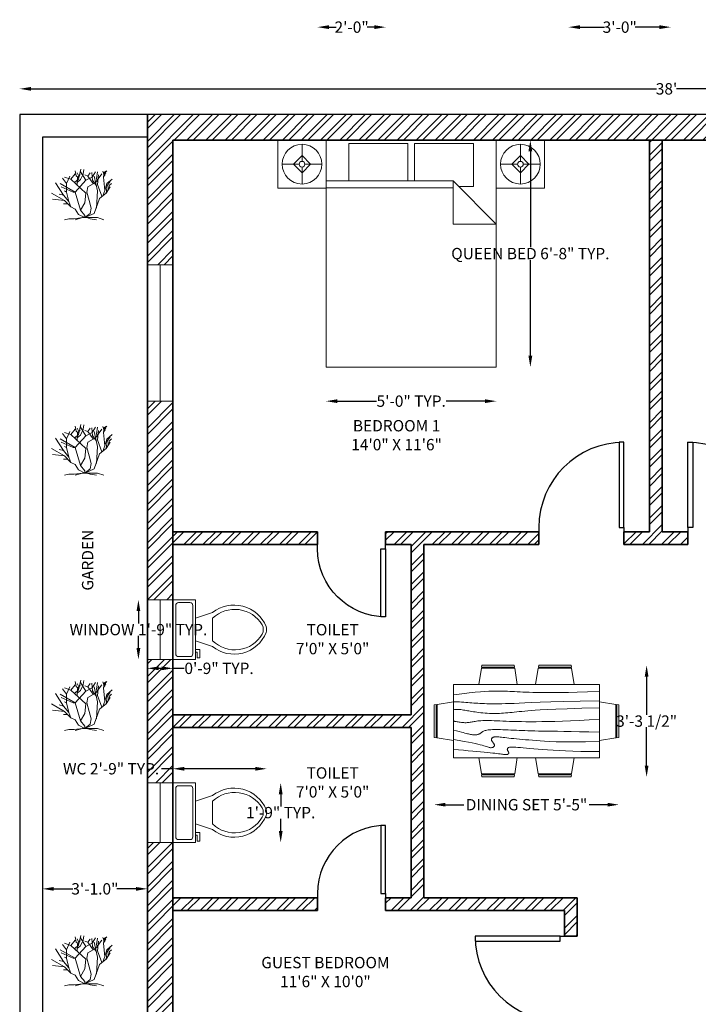
# Model space of a CAD drawing. Units: inches. Extents: x 0 to 478, y -33 to 633.
# Tile 3 of 4: x 0 to 239, y 286 to 633. Entities that reach past the tile are written whole.
import ezdxf

# ---------------------------------------------------------------- set-up
doc = ezdxf.new("R2010")
doc.units = ezdxf.units.IN
for name, color, linetype, lineweight in [('A-ANNO-DIMS', 2, 'Continuous', 18), ('A-AREA-IDEN', 7, 'Continuous', 18), ('A-DOOR', 3, 'Continuous', 25), ('A-FLOR-FIXT', 9, 'Continuous', 18), ('A-FURN', 8, 'Continuous', 18), ('A-GLAZ', 4, 'Continuous', 18), ('A-WALL', 7, 'Continuous', 35), ('A-WALL-PATT', 252, 'Continuous', 13), ('C-PROP', 7, 'Continuous', 30), ('L-PLNT', 3, 'Continuous', 18)]:
    doc.layers.add(name, color=color, linetype=linetype, lineweight=lineweight)
doc.styles.get("Standard").update_dxf_attribs({"font": 'arial.ttf'})
doc.dimstyles.get("Standard").update_dxf_attribs({"dimtxt": 4, "dimasz": 4, "dimexe": 0.18, "dimexo": 0.0625, "dimgap": 0.09, "dimtad": 0, "dimtih": 1, "dimtoh": 1, "dimdec": 1, "dimzin": 0, "dimdsep": 46, "dimlunit": 3, "dimtxsty": 'Standard', "dimcen": 0.09, "dimse1": 1, "dimse2": 1, "dimadec": 0, "dimazin": 0, "dimtfac": 1, "dimtdec": 1, "dimtofl": 0, "dimtmove": 0, "dimatfit": 3, "dimfxl": 1, "dimtolj": 1, "dimtzin": 0, "dimarcsym": 0})

# ---------------------------------------------------------------- blocks, each defined once
blk = doc.blocks.new('Dining Set - 36 x 72 in.')
for p, q in [((-22.2343, 26.00059), (-23.4847, 17.99762)), ((-22.2304, 26), (-5.7608, 26)), ((-22, 27.5), (-22.1562, 26.50042)), ((-5.8416, 26.5), (-22.1534, 26.5)), ((-22, 27.5), (-6, 27.5)), ((-5.8437, 26.49966), (-6, 27.5)), ((-4.5152, 17.99762), (-5.7655, 25.99926)), ((5.7657, 26.00059), (4.5153, 17.99762)), ((5.7696, 26), (22.2392, 26)), ((6, 27.5), (5.8438, 26.50042)), ((22.1584, 26.5), (5.8466, 26.5)), ((6, 27.5), (22, 27.5)), ((22.1563, 26.49966), (22, 27.5)), ((23.4848, 17.99762), (22.2345, 25.99926)), ((36, 18), (-36, 18)), ((-36, 18), (-36, -18)), ((36, -18), (36, 18)), ((-45.5, 8), (-44.5004, 8.15617)), ((-45.5, 8), (-45.5, -8)), ((-44.5, -8.15843), (-44.5, 8.15338)), ((-44.0006, 8.23428), (-35.9976, 9.48474)), ((-44, 8.23041), (-44, -8.23915)), ((44.0006, 8.23428), (35.9976, 9.48474)), ((44, 8.23041), (44, -8.23915)), ((44.5, -8.15843), (44.5, 8.15338)), ((45.5, 8), (44.5005, 8.15617)), ((45.5, 8), (45.5, -8)), ((-44.4997, -8.15631), (-45.5, -8)), ((-35.9976, -9.48476), (-43.9993, -8.2345)), ((35.9976, -9.48476), (43.9993, -8.2345)), ((44.4997, -8.15631), (45.5, -8)), ((-36, -18), (36, -18)), ((-22.2343, -26.0006), (-23.4847, -17.99762)), ((-4.5152, -17.99762), (-5.7655, -25.99928)), ((5.7657, -26.0006), (4.5153, -17.99762)), ((23.4848, -17.99762), (22.2345, -25.99928)), ((-22.2304, -26), (-5.7608, -26)), ((-22, -27.5), (-22.1562, -26.50044)), ((-5.8416, -26.5), (-22.1534, -26.5)), ((-22, -27.5), (-6, -27.5)), ((-5.8437, -26.49967), (-6, -27.5)), ((5.7696, -26), (22.2392, -26)), ((6, -27.5), (5.8438, -26.50044)), ((22.1584, -26.5), (5.8466, -26.5)), ((6, -27.5), (22, -27.5)), ((22.1563, -26.49967), (22, -27.5))]:
    blk.add_line(p, q)
for points in [[(-36, 15), (-31.1772, 14.97754), (-26.8079, 14.91406), (-22.8538, 14.81543), (-19.276, 14.6875), (-16.0362, 14.53613), (-13.0957, 14.36718), (-10.4159, 14.18652), (-7.9583, 14), (-5.6904, 13.81315), (-3.6035, 13.63021), (-1.6954, 13.45508), (0.0365, 13.29166), (1.5945, 13.14388), (2.9811, 13.01562), (4.1988, 12.9108), (5.25, 12.83333), (6.1393, 12.78613), (6.8802, 12.76823), (7.4883, 12.77767), (7.9792, 12.8125), (8.3685, 12.87077), (8.6719, 12.95052), (8.9049, 13.0498), (9.0833, 13.16666), (9.2205, 13.29899), (9.3216, 13.44401), (9.3895, 13.59879), (9.4271, 13.76041), (9.4373, 13.92594), (9.4232, 14.09245), (9.3875, 14.257), (9.3333, 14.41666), (9.2638, 14.56917), (9.1836, 14.71484), (9.0975, 14.85465), (9.0104, 14.98958), (8.9272, 15.1206), (8.8529, 15.2487), (8.7922, 15.37483), (8.75, 15.5), (8.7305, 15.62467), (8.7344, 15.74739), (8.7617, 15.86621), (8.8125, 15.97916), (8.8867, 16.08431), (8.9844, 16.17968), (9.1055, 16.26334), (9.25, 16.33333), (9.4189, 16.38802), (9.6172, 16.42708), (9.8506, 16.45052), (10.125, 16.45833), (10.4463, 16.45052), (10.8203, 16.42708), (11.2529, 16.38802), (11.75, 16.33333), (12.3184, 16.26318), (12.9694, 16.17838), (13.7151, 16.07991), (14.5677, 15.96875), (15.5395, 15.84586), (16.6426, 15.71224), (17.8893, 15.56884), (19.2917, 15.41666), (20.859, 15.25667), (22.5879, 15.08984), (24.4721, 14.91715), (26.5052, 14.73958), (28.6809, 14.5581), (30.9929, 14.3737), (33.4347, 14.18733), (36, 14)], [(-36, 10), (-28.9766, 10.14274), (-23.1725, 10.20442), (-18.4241, 10.19775), (-14.5677, 10.13541), (-11.4399, 10.03011), (-8.877, 9.89453), (-6.7154, 9.74137), (-4.7917, 9.58333), (-2.9698, 9.43082), (-1.2246, 9.28515), (0.4415, 9.14534), (2.026, 9.01041), (3.5266, 8.87939), (4.9408, 8.7513), (6.266, 8.62516), (7.5, 8.5), (8.6411, 8.37549), (9.6914, 8.2539), (10.6538, 8.13818), (11.5312, 8.03125), (12.3267, 7.93603), (13.043, 7.85547), (13.6831, 7.79248), (14.25, 7.75), (14.7471, 7.7303), (15.1797, 7.73307), (15.5537, 7.75732), (15.875, 7.80208), (16.1494, 7.86637), (16.3828, 7.94922), (16.5811, 8.04964), (16.75, 8.16666), (16.8944, 8.29915), (17.0143, 8.44531), (17.1089, 8.60319), (17.1771, 8.77083), (17.218, 8.94629), (17.2305, 9.1276), (17.2137, 9.31282), (17.1667, 9.5), (17.0895, 9.6875), (16.987, 9.875), (16.8649, 10.0625), (16.7292, 10.25), (16.5856, 10.4375), (16.4401, 10.625), (16.2985, 10.8125), (16.1667, 11), (16.05, 11.18733), (15.9518, 11.3737), (15.8752, 11.5581), (15.8229, 11.73958), (15.798, 11.91715), (15.8034, 12.08984), (15.842, 12.25667), (15.9167, 12.41666), (16.0295, 12.56836), (16.1784, 12.70833), (16.3605, 12.83268), (16.5729, 12.9375), (16.8127, 13.01888), (17.0768, 13.07291), (17.3625, 13.0957), (17.6667, 13.08333), (17.9894, 13.03312), (18.3418, 12.94726), (18.7382, 12.82918), (19.1927, 12.68229), (19.7195, 12.51001), (20.3327, 12.31575), (21.0465, 12.10294), (21.875, 11.875), (22.8357, 11.63354), (23.959, 11.37304), (25.2786, 11.08618), (26.8282, 10.76562), (28.6414, 10.40405), (30.752, 9.99414), (33.1936, 9.52856), (36, 9)], [(-36, 5.5), (-30.7157, 5.3348), (-26.069, 5.20963), (-21.9946, 5.11767), (-18.4271, 5.05208), (-15.3009, 5.00602), (-12.5508, 4.97265), (-10.1112, 4.94515), (-7.9167, 4.91666), (-5.909, 4.88167), (-4.0586, 4.83984), (-2.3429, 4.79215), (-0.7396, 4.73958), (0.7739, 4.6831), (2.22, 4.6237), (3.6213, 4.56233), (5, 4.5), (6.373, 4.43782), (7.7344, 4.3776), (9.0723, 4.32129), (10.375, 4.27083), (11.6309, 4.22819), (12.8281, 4.19531), (13.9551, 4.17415), (15, 4.16666), (15.954, 4.17448), (16.819, 4.19791), (17.6001, 4.23698), (18.3021, 4.29166), (18.9299, 4.36198), (19.4883, 4.44791), (19.9823, 4.54948), (20.4167, 4.66666), (20.7969, 4.79899), (21.1302, 4.94401), (21.4245, 5.09879), (21.6875, 5.26041), (21.9271, 5.42594), (22.1511, 5.59245), (22.3672, 5.757), (22.5834, 5.91666), (22.8065, 6.06868), (23.0404, 6.21093), (23.2879, 6.34147), (23.5521, 6.45833), (23.8358, 6.55957), (24.142, 6.64323), (24.4735, 6.70735), (24.8334, 6.75), (25.2235, 6.76969), (25.642, 6.76692), (26.0858, 6.74267), (26.5521, 6.69791), (27.0379, 6.63362), (27.5404, 6.55078), (28.0565, 6.45036), (28.5834, 6.33333), (29.1242, 6.19987), (29.7071, 6.04687), (30.3661, 5.87044), (31.1354, 5.66666), (32.0493, 5.43164), (33.142, 5.16146), (34.4475, 4.85221), (36, 4.5)], [(-36, -1), (-30.7915, -0.6591), (-26.0195, -0.38216), (-21.6519, -0.16284), (-17.6563, 0.00521), (-14.0005, 0.12833), (-10.6523, 0.21289), (-7.5796, 0.26522), (-4.75, 0.29166), (-2.134, 0.29793), (0.2878, 0.28711), (2.5317, 0.26163), (4.6146, 0.22396), (6.5529, 0.17651), (8.3633, 0.12174), (10.0623, 0.06209), (11.6667, 0), (13.1899, -0.06201), (14.6341, -0.1211), (15.9982, -0.17432), (17.2813, -0.21875), (18.4823, -0.25147), (19.6003, -0.26953), (20.6343, -0.27002), (21.5834, -0.25), (22.4481, -0.20768), (23.2357, -0.14584), (23.9549, -0.06836), (24.6146, 0.02083), (25.2235, 0.11784), (25.7904, 0.21875), (26.3241, 0.31966), (26.8334, 0.41666), (27.3265, 0.50618), (27.8099, 0.58593), (28.2894, 0.65397), (28.7709, 0.70833), (29.2601, 0.74707), (29.763, 0.76823), (30.2855, 0.76985), (30.8334, 0.75), (31.4088, 0.70784), (31.9994, 0.64713), (32.589, 0.57275), (33.1615, 0.48958), (33.7008, 0.4025), (34.1908, 0.3164), (34.6153, 0.23616), (34.9584, 0.16666), (35.2099, 0.11165), (35.3848, 0.07031), (35.504, 0.04069), (35.5886, 0.02083), (35.6594, 0.00879), (35.7377, 0.0026), (35.8442, 0.00032), (36, 0)], [(-36, -6.5), (-27.1843, -6.31267), (-20.084, -6.1263), (-14.469, -5.9419), (-10.1094, -5.76042), (-6.7752, -5.58285), (-4.2363, -5.41016), (-2.2629, -5.24333), (-0.625, -5.08334), (0.8708, -4.93099), (2.2715, -4.78646), (3.5872, -4.64974), (4.8281, -4.52084), (6.0046, -4.39974), (7.127, -4.28646), (8.2053, -4.18099), (9.25, -4.08334), (10.2705, -3.99382), (11.2734, -3.91407), (12.2647, -3.84603), (13.25, -3.79167), (14.2354, -3.75293), (15.2266, -3.73177), (16.2295, -3.73015), (17.25, -3.75), (18.2912, -3.79248), (19.3451, -3.85547), (20.4009, -3.93604), (21.4479, -4.03125), (22.4754, -4.13819), (23.4727, -4.25391), (24.4289, -4.37549), (25.3334, -4.5), (26.1785, -4.62492), (26.9694, -4.74935), (27.7145, -4.87281), (28.4219, -4.99479), (29.1, -5.11483), (29.7572, -5.23242), (30.4016, -5.34709), (31.0417, -5.45834), (31.6837, -5.56437), (32.3262, -5.65821), (32.9658, -5.73153), (33.599, -5.77604), (34.2224, -5.78345), (34.8327, -5.74545), (35.4264, -5.65373), (36, -5.5)], [(-36, -10), (-26.4022, -9.81299), (-18.4675, -9.62891), (-11.9839, -9.45069), (-6.7396, -9.28125), (-2.5226, -9.12354), (0.8789, -8.98047), (3.6769, -8.85498), (6.0833, -8.75), (8.2767, -8.66765), (10.3021, -8.60677), (12.1712, -8.56543), (13.8958, -8.54167), (15.4876, -8.53353), (16.9583, -8.53907), (18.3197, -8.55632), (19.5834, -8.58334), (20.7616, -8.61841), (21.8685, -8.66081), (22.9188, -8.71004), (23.9271, -8.76563), (24.9081, -8.82707), (25.8763, -8.89388), (26.8465, -8.96558), (27.8334, -9.04167), (28.8474, -9.12118), (29.8828, -9.20117), (30.93, -9.27824), (31.9792, -9.34896), (33.0205, -9.40991), (34.0443, -9.45768), (35.0407, -9.48885), (36, -9.5)], [(-36, -14.5), (-30.0881, -14.33513), (-25.0332, -14.21224), (-20.7312, -14.12647), (-17.0781, -14.07292), (-13.97, -14.04671), (-11.3027, -14.04297), (-8.9724, -14.05681), (-6.875, -14.08334), (-4.9224, -14.11833), (-3.0905, -14.16016), (-1.3709, -14.20785), (0.2448, -14.26042), (1.7647, -14.3169), (3.1973, -14.3763), (4.5507, -14.43767), (5.8333, -14.5), (7.0554, -14.5621), (8.235, -14.62175), (9.3922, -14.67652), (10.5469, -14.72396), (11.7192, -14.76164), (12.929, -14.78711), (14.1965, -14.79794), (15.5417, -14.79167), (16.9933, -14.76424), (18.6152, -14.70508), (20.4804, -14.60197), (22.6615, -14.44271), (25.2312, -14.21509), (28.2624, -13.9069), (31.8277, -13.50594), (36, -13)]]:
    blk.add_lwpolyline(points)
blk = doc.blocks.new('Bed - Queen')
for p, q in [((0, -80.00003), (0, 0)), ((0, 0), (59.99999, 0)), ((59.99999, 0), (59.99999, -80.00003)), ((7.99999, -1.2), (28.79998, -1.2)), ((7.99999, -14.4), (7.99999, -1.2)), ((28.79998, -1.2), (28.79998, -14.4)), ((31.19999, -1.2), (51.99999, -1.2)), ((31.19999, -14.4), (31.19999, -1.2)), ((51.99999, -1.2), (51.99999, -16.4)), ((0, -14.4), (44.8, -14.4)), ((44.8, -16.8), (0, -16.8)), ((59.99999, -29.6), (44.8, -14.4)), ((44.8, -14.4), (44.8, -29.6)), ((51.99999, -16.4), (46.79936, -16.4)), ((44.8, -29.6), (59.99999, -29.6)), ((59.99999, -80.00003), (0, -80.00003))]:
    blk.add_line(p, q)
blk = doc.blocks.new('Toilet - top')
for p, q in [((9.5, -6), (9.5, -2)), ((-10, -8.5), (-8, -8.5)), ((-10, -9.5), (-10, -8.5)), ((-7, -9.5), (-10, -9.5)), ((-8, -8.5), (-8, -8)), ((-7, -8), (-7, -9.5)), ((-4, -8), (-6, -14)), ((4, -8), (6, -14)), ((4, -14), (-4, -14))]:
    blk.add_line(p, q)
blk.add_lwpolyline([(10.5, -8), (10.5, 0), (-10.5, 0), (-10.5, -8)], close=True)
for points in [[(-9.5, -2), (-9.5, -6)], [(8.5, -1), (-8.5, -1)], [(-8.5, -7), (8.5, -7)]]:
    blk.add_lwpolyline(points)
for centre, radius, start, end in [((-8.62, -1.88), 0.884, 81.8699, 188.1301), ((8.62, -1.88), 0.884, 351.8699, 98.1301), ((-8.62, -6.12), 0.884, 171.8699, 278.1301), ((8.62, -6.12), 0.884, 261.8699, 8.1301), ((3.52, -21.58), 12.17, 141.4691, 247.9714), ((4.2, -21.82), 11.33, 136.3677, 238.9468), ((-3.52, -21.58), 12.17, 292.0284, 38.5307), ((-4.2, -21.82), 11.33, 301.053, 43.6321), ((0, -27.88), 4, 245.7318, 294.2682), ((0, -29), 4, 254.8605, 285.1395)]:
    blk.add_arc(centre, radius, start, end)
blk = doc.blocks.new('*U11')
for p, q in [((0, 0), (0, -6)), ((30, 0), (30, -6))]:
    blk.add_line(p, q)
blk.add_lwpolyline([(0, 0), (0, 30), (1.75, 30), (1.75, 0)], close=True)
blk.add_arc((0, 0), 30, 0, 90)
blk = doc.blocks.new('*U12')
for p, q in [((-30, 0), (-30, -6)), ((0, 0), (0, -6))]:
    blk.add_line(p, q)
blk.add_lwpolyline([(0, 0), (0, 30), (-1.75, 30), (-1.75, 0)], close=True)
blk.add_arc((0, 0), 30, 90, 180)
blk = doc.blocks.new('*U13')
for p, q in [((-24, 0), (-24, -6)), ((0, 0), (0, -6))]:
    blk.add_line(p, q)
blk.add_lwpolyline([(0, 0), (0, 24), (-1.75, 24), (-1.75, 0)], close=True)
blk.add_arc((0, 0), 24, 90, 180)
blk = doc.blocks.new('*U15')
for p, q in [((-30, 0), (-30, -6)), ((0, 0), (0, -6))]:
    blk.add_line(p, q)
blk.add_lwpolyline([(0, 0), (0, 30), (-1.75, 30), (-1.75, 0)], close=True)
blk.add_arc((0, 0), 30, 90, 180)
blk = doc.blocks.new('Shrub - elevation')
for p, q in [((-11.433, 18.289), (-10.457, 22.749)), ((-9.48, 19.775), (-8.992, 22.592)), ((-16.8, 16.32), (-18.72, 18.72)), ((-14.88, 18.24), (-17.76, 19.2)), ((-16.8, 16.32), (-15.36, 19.68)), ((-14.88, 18.24), (-12.96, 20.64)), ((-8.16, 12), (-14.88, 18.24)), ((-13.325, 16.724), (-11.433, 18.289)), ((-12.96, 12.48), (-8.16, 17.76)), ((-12.471, 19.775), (-12.898, 22.044)), ((-11.677, 19.071), (-12.471, 19.775)), ((-11.28, 19.619), (-12.104, 21.184)), ((-12.043, 15.628), (-11.921, 18.836)), ((-11.982, 16.802), (-10.579, 18.054)), ((-11.921, 18.836), (-10.64, 20.401)), ((-10.579, 18.054), (-9.846, 19.697)), ((-8.16, 17.76), (-10.56, 21.6)), ((-7.2, 19.68), (-8.64, 20.16)), ((-8.16, 17.76), (-5.28, 19.2)), ((-7.2, 19.68), (-6.24, 21.12)), ((-4.8, 16.32), (-7.2, 19.68)), ((-5.086, 17.741), (-5.513, 21.34)), ((-5.28, 19.2), (-3.84, 21.6)), ((-3.377, 15.315), (-5.086, 17.819)), ((-2.88, 12.96), (-4.32, 19.68)), ((-3.84, 16.8), (-0.96, 20.64)), ((-3.377, 18.602), (-2.888, 21.575)), ((-2.766, 16.802), (-3.377, 18.602)), ((-2.88, 15.84), (-2.4, 20.16)), ((-0.508, 21.888), (-0.081, 20.558)), ((-0.203, 19.149), (0.102, 21.34)), ((0.346, 13.203), (-0.203, 19.149)), ((-0.142, 19.384), (0.59, 20.401)), ((-0.02, 20.01), (0.896, 21.105)), ((0.041, 20.714), (1.384, 22.044)), ((0.102, 21.34), (0.835, 21.888)), ((1.323, 16.254), (3.642, 18.289)), ((-18.24, 11.04), (-21.755, 16.655)), ((-12.96, 12.48), (-19.68, 16.32)), ((-13.92, 12.48), (-19.2, 14.88)), ((-16.8, 12.48), (-16.8, 16.32)), ((-7.68, 12.48), (-7.2, 14.88)), ((-7.2, 14.88), (-3.84, 16.8)), ((-0.96, 10.56), (-2.88, 15.84)), ((0.346, 13.203), (1.323, 16.254)), ((0.96, 12), (1.44, 15.36)), ((0.96, 12), (2.88, 14.88)), ((1.44, 15.36), (2.88, 17.28)), ((1.92, 13.44), (2.4, 15.36)), ((2.4, 15.36), (3.36, 16.32)), ((-17.76, 8.64), (-23.663, 11.961)), ((-17.76, 8.64), (-23.128, 9.222)), ((-18.24, 11.04), (-20.16, 11.52)), ((-15.84, 8.16), (-18.24, 11.04)), ((-16.8, 12.48), (-17.76, 12.96)), ((-15.84, 8.16), (-16.8, 12.48)), ((-12.96, 12.48), (-13.92, 12.48)), ((-10.56, 4.32), (-12.96, 12.48)), ((-8.64, 7.68), (-8.16, 12)), ((-6.72, 8.64), (-7.68, 12.48)), ((-4.32, 2.88), (-1.92, 9.6)), ((-3.36, 5.28), (-2.88, 12.96)), ((-1.92, 9.6), (0.96, 12)), ((-0.48, 10.8), (0.346, 13.203)), ((-16.32, 7.2), (-18.24, 7.2)), ((-14.88, 5.76), (-17.76, 8.64)), ((-14.88, 5.76), (-15.84, 8.16)), ((-12.96, 4.8), (-14.88, 5.76)), ((-11.52, 2.4), (-12.96, 4.8)), ((-10.56, 4.32), (-8.64, 7.68)), ((-5.76, 5.28), (-6.72, 8.64)), ((-6.24, 2.88), (-5.76, 5.28)), ((-15.84, 0.48), (-17.76, 0)), ((-13.44, 0.48), (-15.84, 0.48)), ((-9.6, 0.96), (-13.44, 0.48)), ((-9.6, 0.96), (-12.96, 0)), ((-8.64, 0.96), (-11.52, 2.4)), ((-8.64, 1.92), (-10.56, 4.32)), ((-9.6, 0.96), (-7.68, 0.96)), ((-8.64, 0.96), (-4.32, 2.88)), ((-8.64, 0.96), (-6.24, 2.88)), ((-8.64, 0.96), (-8.64, 1.92)), ((-8.64, 0.96), (-2.88, 0.96)), ((-7.68, 0.96), (-6.24, 0.48)), ((-6.24, 0.48), (-3.36, 0)), ((-2.88, 0.96), (0, 0))]:
    blk.add_line(p, q)
blk = doc.blocks.new('*D22')
at = {"layer": 'A-ANNO-DIMS', "color": 0, "lineweight": -2, "transparency": 16777216}
for p, q in [((12, 327.14), (18.76, 327.14)), ((41, 327.14), (34.24, 327.14))]:
    blk.add_line(p, q, dxfattribs=at)
at = {"layer": 'A-ANNO-DIMS', "color": 0, "transparency": 16777216}
for points in [[(12, 327.8), (12, 326.47), (8, 327.14)], [(41, 327.8), (41, 326.47), (45, 327.14)]]:
    blk.add_solid(points, dxfattribs=at)
at = {"layer": 'Defpoints', "color": 0, "transparency": 16777216}
for p in [(8, 364.5), (45, 364.5), (8, 327.14)]:
    blk.add_point(p, dxfattribs=at)
at = {"layer": 'A-ANNO-DIMS', "color": 0, "transparency": 16777216, "insert": (26.5, 327.14), "char_height": 4, "attachment_point": 5}
blk.add_mtext('\\A1;3\'-1.0"', dxfattribs=at)
blk = doc.blocks.new('*D25')
at = {"layer": 'A-ANNO-DIMS', "color": 0, "lineweight": -2, "transparency": 16777216}
for p, q in [((4, 609.06), (224.52, 609.06)), ((452, 609.06), (231.48, 609.06))]:
    blk.add_line(p, q, dxfattribs=at)
at = {"layer": 'A-ANNO-DIMS', "color": 0, "transparency": 16777216}
for points in [[(4, 609.73), (4, 608.4), (0, 609.06)], [(452, 609.73), (452, 608.4), (456, 609.06)]]:
    blk.add_solid(points, dxfattribs=at)
at = {"layer": 'Defpoints', "color": 0, "transparency": 16777216}
for p in [(0, 609.06), (0, 600), (456, 600)]:
    blk.add_point(p, dxfattribs=at)
at = {"layer": 'A-ANNO-DIMS', "color": 0, "transparency": 16777216, "insert": (228, 609.06), "char_height": 4, "attachment_point": 5}
blk.add_mtext("\\A1;38'", dxfattribs=at)
blk = doc.blocks.new('WIN-48IN')
for p, q in [((0, 48), (9, 48)), ((4.5, 48), (4.5, 0)), ((0, 0), (9, 0))]:
    blk.add_line(p, q)
blk = doc.blocks.new('WIN-21IN')
for p, q in [((0, 9), (0, 0)), ((21, 9), (21, 0)), ((0, 4.5), (21, 4.5))]:
    blk.add_line(p, q)
blk = doc.blocks.new('Lamp - Table')
for p, q in [((0, 7), (0, 1)), ((-1, 0), (-7, 0)), ((0, 3), (-3, 0)), ((-3, 0), (0, -3)), ((3, 0), (0, 3)), ((0, -3), (3, 0)), ((1, 0), (7, 0)), ((0, -1), (0, -7))]:
    blk.add_line(p, q)
for radius in [7, 1]:
    blk.add_circle((0, 0), radius)
blk = doc.blocks.new('END-TABLE-WITH-LAMP')
blk.add_lwpolyline([(-8.49, 8.49), (-8.49, -8.49), (8.49, -8.49), (8.49, 8.49)], close=True)
blk.add_blockref('Lamp - Table', (0, 0))
blk = doc.blocks.new('*D38')
at = {"layer": 'A-ANNO-DIMS', "color": 0, "lineweight": -2, "transparency": 16777216}
for p, q in [((180, 587), (180, 553.28)), ((180, 515), (180, 548.72))]:
    blk.add_line(p, q, dxfattribs=at)
at = {"layer": 'A-ANNO-DIMS', "color": 0, "transparency": 16777216}
for points in [[(179.33, 587), (180.67, 587), (180, 591)], [(179.33, 515), (180.67, 515), (180, 511)]]:
    blk.add_solid(points, dxfattribs=at)
at = {"layer": 'Defpoints', "color": 0, "transparency": 16777216}
for p in [(168, 591), (180, 591), (168, 511)]:
    blk.add_point(p, dxfattribs=at)
at = {"layer": 'A-ANNO-DIMS', "color": 0, "transparency": 16777216, "insert": (180, 551), "char_height": 4, "attachment_point": 5}
blk.add_mtext('\\A1;QUEEN BED 6\'-8" TYP.', dxfattribs=at)
blk = doc.blocks.new('*D39')
at = {"layer": 'A-ANNO-DIMS', "color": 0, "lineweight": -2, "transparency": 16777216}
for p, q in [((112, 499), (125.72, 499)), ((164, 499), (150.28, 499))]:
    blk.add_line(p, q, dxfattribs=at)
at = {"layer": 'A-ANNO-DIMS', "color": 0, "transparency": 16777216}
for points in [[(112, 499.67), (112, 498.33), (108, 499)], [(164, 499.67), (164, 498.33), (168, 499)]]:
    blk.add_solid(points, dxfattribs=at)
at = {"layer": 'Defpoints', "color": 0, "transparency": 16777216}
for p in [(108, 511), (168, 511), (168, 499)]:
    blk.add_point(p, dxfattribs=at)
at = {"layer": 'A-ANNO-DIMS', "color": 0, "transparency": 16777216, "insert": (138, 499), "char_height": 4, "attachment_point": 5}
blk.add_mtext('\\A1;5\'-0" TYP.', dxfattribs=at)
blk = doc.blocks.new('*D40')
at = {"layer": 'A-ANNO-DIMS', "color": 0, "lineweight": -2, "transparency": 16777216}
for p, q in [((54, 369.46), (50, 369.46)), ((83.05, 369.46), (58, 369.46))]:
    blk.add_line(p, q, dxfattribs=at)
at = {"layer": 'A-ANNO-DIMS', "color": 0, "transparency": 16777216}
for points in [[(58, 370.12), (58, 368.79), (54, 369.46)], [(83.05, 370.12), (83.05, 368.79), (87.05, 369.46)]]:
    blk.add_solid(points, dxfattribs=at)
at = {"layer": 'Defpoints', "color": 0, "transparency": 16777216}
for p in [(54, 369.46), (54, 364.5), (87.05, 364.5)]:
    blk.add_point(p, dxfattribs=at)
at = {"layer": 'A-ANNO-DIMS', "color": 0, "transparency": 16777216, "insert": (32.21, 369.46), "char_height": 4, "attachment_point": 5}
blk.add_mtext('\\A1;WC 2\'-9" TYP.', dxfattribs=at)
blk = doc.blocks.new('*D41')
at = {"layer": 'A-ANNO-DIMS', "color": 0, "lineweight": -2, "transparency": 16777216}
for p, q in [((92, 360.5), (92, 356.13)), ((92, 347.5), (92, 351.87))]:
    blk.add_line(p, q, dxfattribs=at)
at = {"layer": 'A-ANNO-DIMS', "color": 0, "transparency": 16777216}
for points in [[(91.34, 360.5), (92.67, 360.5), (92, 364.5)], [(91.34, 347.5), (92.67, 347.5), (92, 343.5)]]:
    blk.add_solid(points, dxfattribs=at)
at = {"layer": 'Defpoints', "color": 0, "transparency": 16777216}
for p in [(87.05, 364.5), (92, 364.5), (87.05, 343.5)]:
    blk.add_point(p, dxfattribs=at)
at = {"layer": 'A-ANNO-DIMS', "color": 0, "transparency": 16777216, "insert": (92, 354), "char_height": 4, "attachment_point": 5}
blk.add_mtext('\\A1;1\'-9" TYP.', dxfattribs=at)
blk = doc.blocks.new('*D42')
at = {"layer": 'A-ANNO-DIMS', "color": 0, "lineweight": -2, "transparency": 16777216}
for p, q in [((41.85, 425), (41.85, 420.66)), ((41.85, 412), (41.85, 416.34))]:
    blk.add_line(p, q, dxfattribs=at)
at = {"layer": 'A-ANNO-DIMS', "color": 0, "transparency": 16777216}
for points in [[(41.18, 425), (42.52, 425), (41.85, 429)], [(41.18, 412), (42.52, 412), (41.85, 408)]]:
    blk.add_solid(points, dxfattribs=at)
at = {"layer": 'Defpoints', "color": 0, "transparency": 16777216}
for p in [(45, 429), (41.85, 408), (45, 408)]:
    blk.add_point(p, dxfattribs=at)
at = {"layer": 'A-ANNO-DIMS', "color": 0, "transparency": 16777216, "insert": (41.85, 418.5), "char_height": 4, "attachment_point": 5}
blk.add_mtext('\\A1;WINDOW 1\'-9" TYP.', dxfattribs=at)
blk = doc.blocks.new('*D43')
at = {"layer": 'A-ANNO-DIMS', "color": 0, "lineweight": -2, "transparency": 16777216}
for p, q in [((49, 404.85), (50, 404.85)), ((54, 404.85), (58, 404.85))]:
    blk.add_line(p, q, dxfattribs=at)
at = {"layer": 'A-ANNO-DIMS', "color": 0, "transparency": 16777216}
for points in [[(49, 405.52), (49, 404.18), (45, 404.85)], [(50, 405.52), (50, 404.18), (54, 404.85)]]:
    blk.add_solid(points, dxfattribs=at)
at = {"layer": 'Defpoints', "color": 0, "transparency": 16777216}
for p in [(45, 408), (54, 408), (54, 404.85)]:
    blk.add_point(p, dxfattribs=at)
at = {"layer": 'A-ANNO-DIMS', "color": 0, "transparency": 16777216, "insert": (70.28, 404.85), "char_height": 4, "attachment_point": 5}
blk.add_mtext('\\A1;0\'-9" TYP.', dxfattribs=at)
blk = doc.blocks.new('*D46')
at = {"layer": 'A-ANNO-DIMS', "color": 0, "lineweight": -2, "transparency": 16777216}
for p, q in [((150.07, 356.8), (156.57, 356.8)), ((207.21, 356.8), (200.71, 356.8))]:
    blk.add_line(p, q, dxfattribs=at)
at = {"layer": 'A-ANNO-DIMS', "color": 0, "transparency": 16777216}
for points in [[(150.07, 357.46), (150.07, 356.13), (146.07, 356.8)], [(207.21, 357.46), (207.21, 356.13), (211.21, 356.8)]]:
    blk.add_solid(points, dxfattribs=at)
at = {"layer": 'Defpoints', "color": 0, "transparency": 16777216}
for p in [(146.07, 366.57), (211.21, 366.57), (146.07, 356.8)]:
    blk.add_point(p, dxfattribs=at)
at = {"layer": 'A-ANNO-DIMS', "color": 0, "transparency": 16777216, "insert": (178.64, 356.8), "char_height": 4, "attachment_point": 5}
blk.add_mtext('\\A1;DINING SET 5\'-5"', dxfattribs=at)
blk = doc.blocks.new('*D47')
at = {"layer": 'A-ANNO-DIMS', "color": 0, "lineweight": -2, "transparency": 16777216}
for p, q in [((220.98, 401.93), (220.98, 388.41)), ((220.98, 370.57), (220.98, 384.09))]:
    blk.add_line(p, q, dxfattribs=at)
at = {"layer": 'A-ANNO-DIMS', "color": 0, "transparency": 16777216}
for points in [[(220.31, 401.93), (221.64, 401.93), (220.98, 405.93)], [(220.31, 370.57), (221.64, 370.57), (220.98, 366.57)]]:
    blk.add_solid(points, dxfattribs=at)
at = {"layer": 'Defpoints', "color": 0, "transparency": 16777216}
for p in [(211.21, 405.93), (211.21, 366.57), (220.98, 366.57)]:
    blk.add_point(p, dxfattribs=at)
at = {"layer": 'A-ANNO-DIMS', "color": 0, "transparency": 16777216, "insert": (220.98, 386.25), "char_height": 4, "attachment_point": 5}
blk.add_mtext('\\A1;3\'-3 1/2"', dxfattribs=at)
blk = doc.blocks.new('*D55')
at = {"layer": 'A-ANNO-DIMS', "color": 0, "lineweight": -2, "transparency": 16777216}
for p, q in [((197.5, 630.8), (206.09, 630.8)), ((225.5, 630.8), (216.91, 630.8))]:
    blk.add_line(p, q, dxfattribs=at)
at = {"layer": 'A-ANNO-DIMS', "color": 0, "transparency": 16777216}
for points in [[(197.5, 631.47), (197.5, 630.13), (193.5, 630.8)], [(225.5, 631.47), (225.5, 630.13), (229.5, 630.8)]]:
    blk.add_solid(points, dxfattribs=at)
at = {"layer": 'Defpoints', "color": 0, "transparency": 16777216}
for p in [(229.5, 630.8), (193.5, 154.5), (229.5, 154.5)]:
    blk.add_point(p, dxfattribs=at)
at = {"layer": 'A-ANNO-DIMS', "color": 0, "transparency": 16777216, "insert": (211.5, 630.8), "char_height": 4, "attachment_point": 5}
blk.add_mtext('\\A1;3\'-0"', dxfattribs=at)
blk = doc.blocks.new('*D56')
at = {"layer": 'A-ANNO-DIMS', "color": 0, "lineweight": -2, "transparency": 16777216}
for p, q in [((109, 630.8), (111.56, 630.8)), ((125, 630.8), (122.44, 630.8))]:
    blk.add_line(p, q, dxfattribs=at)
at = {"layer": 'A-ANNO-DIMS', "color": 0, "transparency": 16777216}
for points in [[(109, 631.47), (109, 630.13), (105, 630.8)], [(125, 631.47), (125, 630.13), (129, 630.8)]]:
    blk.add_solid(points, dxfattribs=at)
at = {"layer": 'Defpoints', "color": 0, "transparency": 16777216}
for p in [(129, 630.8), (105, 453), (129, 453)]:
    blk.add_point(p, dxfattribs=at)
at = {"layer": 'A-ANNO-DIMS', "color": 0, "transparency": 16777216, "insert": (117, 630.8), "char_height": 4, "attachment_point": 5}
blk.add_mtext('\\A1;2\'-0"', dxfattribs=at)
blk = doc.blocks.new('*D57')
at = {"layer": 'A-ANNO-DIMS', "color": 0, "lineweight": -2, "transparency": 16777216}
for p, q in [((239.5, -30.8), (245.06, -30.8)), ((261.5, -30.8), (255.94, -30.8))]:
    blk.add_line(p, q, dxfattribs=at)
at = {"layer": 'A-ANNO-DIMS', "color": 0, "transparency": 16777216}
for points in [[(239.5, -30.13), (239.5, -31.47), (235.5, -30.8)], [(261.5, -30.13), (261.5, -31.47), (265.5, -30.8)]]:
    blk.add_solid(points, dxfattribs=at)
at = {"layer": 'Defpoints', "color": 0, "transparency": 16777216}
for p in [(235.5, 448.5), (265.5, 448.5), (265.5, -30.8)]:
    blk.add_point(p, dxfattribs=at)
at = {"layer": 'A-ANNO-DIMS', "color": 0, "transparency": 16777216, "insert": (250.5, -30.8), "char_height": 4, "attachment_point": 5}
blk.add_mtext('\\A1;2\'-6"', dxfattribs=at)

msp = doc.modelspace()

# ---------------------------------------------------------------- hatches: boundary and pattern name
at = {"layer": 'A-WALL-PATT'}
h = msp.add_hatch(dxfattribs=at)
h.set_pattern_fill('ANSI32', color=256, scale=0.5)
h.paths.add_polyline_path([(456, 600), (45, 600), (45, 547.04), (54, 547.04), (54, 591), (447, 591), (447, 507), (433.5, 507), (433.5, 498), (456, 498)])
h.paths.add_polyline_path([(54, 499.04), (45, 499.04), (45, 429), (54, 429)])
h.paths.add_polyline_path([(235.5, 453), (226.5, 453), (226.5, 591), (222, 591), (222, 453), (213, 453), (213, 448.5), (235.5, 448.5)])
h.paths.add_polyline_path([(105, 453), (54, 453), (54, 448.5), (105, 448.5)], flags=17)
h.paths.add_polyline_path([(183, 453), (129, 453), (129, 448.5), (138, 448.5), (138, 388.5), (54, 388.5), (54, 384), (138, 384), (138, 324), (129, 324), (129, 319.5), (192, 319.5), (192, 310.5), (196.5, 310.5), (196.5, 324), (142.5, 324), (142.5, 448.5), (183, 448.5)])
h.paths.add_polyline_path([(403.5, 453), (265.5, 453), (265.5, 448.5), (394.5, 448.5), (394.5, 442.5), (397.5, 442.5), (403.5, 442.5)])
h.paths.add_polyline_path([(412.5, 507), (399, 507), (399, 558), (394.5, 558), (394.5, 498), (412.5, 498)], flags=17)
h.paths.add_polyline_path([(399, 591), (394.5, 591), (394.5, 582), (399, 582)], flags=17)
h.paths.add_polyline_path([(54, 408), (45, 408), (45, 364.5), (54, 364.5)])
h.paths.add_polyline_path([(54, 343.5), (45, 343.5), (45, 275.82), (54, 275.82), (54, 319.5)])
h.paths.add_polyline_path([(105, 324), (54, 324), (54, 319.5), (105, 319.5)], flags=17)
h.paths.add_polyline_path([(403.5, 412.5), (397.5, 412.5), (394.5, 412.5), (394.5, 388.53), (403.5, 388.53)])
h.paths.add_polyline_path([(403.5, 340.53), (394.5, 340.53), (394.5, 311.5), (256.5, 311.5), (256.5, 307), (394.5, 307), (394.5, 255.85), (403.5, 255.85)])
h.paths.add_polyline_path([(54, 216.47), (54, 227.82), (45, 227.82), (45, 190.5), (95.47, 190.5), (95.47, 199.5), (70.97, 199.5), (54, 199.5)])
h.paths.add_polyline_path([(196.5, 280.5), (192, 280.5), (192, 199.5), (143.47, 199.5), (143.47, 190.5), (187.5, 190.5), (187.5, 188.75), (193.5, 188.75), (196.5, 188.75)])
h.paths.add_polyline_path([(403.5, 207.85), (394.5, 207.85), (394.5, 126.5), (403.5, 126.5)])
h.paths.add_polyline_path([(403.5, 78.5), (394.5, 78.5), (394.5, 63), (265.7, 63), (265.7, 54), (403.5, 54)])
h.paths.add_polyline_path([(394.5, 151), (313.7, 151), (313.7, 142), (394.5, 142)])
h.paths.add_polyline_path([(265.7, 151), (196.5, 151), (196.5, 152.75), (193.5, 152.75), (187.5, 152.75), (187.5, 142), (265.7, 142)])

# ---------------------------------------------------------------- linework, layer by layer
at = {"layer": 'A-WALL'}
for p, q in [((45, 600), (45, 190.5)), ((447, 591), (54, 591)), ((54, 591), (54, 199.5)), ((222, 591), (222, 453)), ((226.5, 591), (226.5, 453)), ((105, 453), (54, 453)), ((105, 448.5), (105, 453)), ((183, 453), (129, 453)), ((129, 448.5), (129, 453)), ((183, 453), (183, 448.5)), ((222, 453), (213, 453)), ((213, 453), (213, 448.5)), ((235.5, 453), (226.5, 453)), ((235.5, 453), (235.5, 448.5)), ((105, 448.5), (54, 448.5)), ((138, 448.5), (129, 448.5)), ((138, 448.5), (138, 388.5)), ((183, 448.5), (142.5, 448.5)), ((142.5, 448.5), (142.5, 324)), ((235.5, 448.5), (213, 448.5)), ((138, 388.5), (54, 388.5)), ((138, 384), (54, 384)), ((138, 384), (138, 324)), ((105, 324), (54, 324)), ((105, 319.5), (105, 324)), ((138, 324), (129, 324)), ((129, 319.5), (129, 324)), ((196.5, 324), (142.5, 324)), ((196.5, 324), (196.5, 310.5)), ((105, 319.5), (54, 319.5)), ((54, 319.5), (54, 199.5)), ((192, 319.5), (129, 319.5)), ((192, 319.5), (192, 310.5)), ((192, 310.5), (196.5, 310.5))]:
    msp.add_line(p, q, dxfattribs=at)
at = {"layer": 'C-PROP'}
for p, q in [((456, 600), (0, 600)), ((0, 600), (0, 0)), ((45, 592), (8, 592)), ((8, 592), (8, 8))]:
    msp.add_line(p, q, dxfattribs=at)

# ---------------------------------------------------------------- block references
at = {"layer": 'A-DOOR'}
for name, p in [('*U12', (213, 454.5)), ('*U11', (235.5, 454.5)), ('*U13', (129, 325.5))]:
    msp.add_blockref(name, p, dxfattribs=at)
at = {"layer": 'A-DOOR', "xscale": -1, "rotation": 180}
msp.add_blockref('*U13', (129, 447), dxfattribs=at)
at = {"layer": 'A-DOOR', "rotation": 90.00000000000003}
msp.add_blockref('*U15', (190.5, 310.5), dxfattribs=at)
at = {"layer": 'A-FLOR-FIXT', "rotation": 89.99999999999999}
for p in [(54, 418.5), (54, 354)]:
    msp.add_blockref('Toilet - top', p, dxfattribs=at)
at = {"layer": 'A-FURN'}
for name, p in [('END-TABLE-WITH-LAMP', (99.51, 582.51)), ('Bed - Queen', (108, 591))]:
    msp.add_blockref(name, p, dxfattribs=at)
at = {"layer": 'A-FURN', "extrusion": (0, 0, -1), "zscale": -1}
msp.add_blockref('END-TABLE-WITH-LAMP', (-176.49, 582.51), dxfattribs=at)
at = {"layer": 'A-FURN', "xscale": 0.7157687565965061, "yscale": 0.7157687565965061, "zscale": 0.7157687565965061, "rotation": 180}
msp.add_blockref('Dining Set - 36 x 72 in.', (178.64, 386.25), dxfattribs=at)
at = {"layer": 'A-GLAZ'}
msp.add_blockref('WIN-48IN', (45, 499.04), dxfattribs=at)
at = {"layer": 'A-GLAZ', "rotation": 270}
for p in [(45, 429), (45, 364.5)]:
    msp.add_blockref('WIN-21IN', p, dxfattribs=at)
at = {"layer": 'L-PLNT', "xscale": 0.78234725202095, "yscale": 0.78234725202095, "zscale": 0.78234725202095}
for p in [(29.69, 562.93), (29.69, 472.93), (29.69, 382.93), (29.69, 292.93)]:
    msp.add_blockref('Shrub - elevation', p, dxfattribs=at)

# ---------------------------------------------------------------- texts
at = {"layer": 'A-AREA-IDEN', "ltscale": 0.5, "char_height": 4, "attachment_point": 1}
for s, width, insert in [('\\pxqc;BEDROOM 1\\P14\'0" X 11\'6"', 37.7397, (113.98, 492.34)), ('\\pxqc;TOILET\\P7\'0" X 5\'0"', 37.7397, (91.44, 420.46)), ('\\pxqc;TOILET\\P7\'0" X 5\'0"', 37.7397, (91.44, 369.98)), ('\\pxqc;GUEST BEDROOM\\P11\'6" X 10\'0"', 50.4232, (82.55, 303.15))]:
    msp.add_mtext_dynamic_manual_height_columns(s, width=width, gutter_width=12.5, heights=[0], dxfattribs=dict(at, insert=insert))
at = {"layer": 'A-AREA-IDEN', "ltscale": 0.5, "insert": (21.95, 424.1), "char_height": 4, "attachment_point": 1, "rotation": 90}
msp.add_mtext_dynamic_manual_height_columns('\\pxqc;GARDEN', width=37.7397, gutter_width=12.5, heights=[0], dxfattribs=at)

# ---------------------------------------------------------------- dimensions: what is measured, and where the dimension line sits
at = {"layer": 'A-ANNO-DIMS'}
for base, p1, p2, override, picture, middle in [((129, 630.8), (105, 453), (129, 453), {"dimdec": 1, "dimlfac": 1, "dimrnd": 0, "dimzin": 1, "dimdsep": 46, "dimlunit": 4, "dimfrac": 2}, '*D56', (117, 630.8)), ((229.5, 630.8), (193.5, 154.5), (229.5, 154.5), {"dimdec": 1, "dimlfac": 1, "dimrnd": 0, "dimzin": 1, "dimdsep": 46, "dimlunit": 4, "dimfrac": 2}, '*D55', (211.5, 630.8)), ((0, 609.06), (456, 600), (0, 600), {"dimclrd": 0, "dimclre": 0, "dimclrt": 0}, '*D25', (228, 609.06)), ((265.5, -30.8), (235.5, 448.5), (265.5, 448.5), {"dimdec": 1, "dimlfac": 1, "dimrnd": 0, "dimzin": 1, "dimdsep": 46, "dimlunit": 4, "dimfrac": 2}, '*D57', (250.5, -30.8)), ((8, 327.14), (45, 364.5), (8, 364.5), {"dimclrd": 0, "dimclre": 0, "dimclrt": 0}, '*D22', (26.5, 327.14))]:
    dim = msp.add_linear_dim(base=base, p1=p1, p2=p2, dimstyle='Standard', override=override, dxfattribs=at)
    dim.commit()
    dim.dimension.update_dxf_attribs({"geometry": picture, "text_midpoint": middle})
for base, p1, p2, angle, text, picture, middle in [((180, 591), (168, 511), (168, 591), 90, 'QUEEN BED <> TYP.', '*D38', (180, 551)), ((41.85, 408), (45, 429), (45, 408), 270, 'WINDOW <> TYP.', '*D42', (41.85, 418.5)), ((54, 369.4569), (87.0462, 364.5), (54, 364.5), 180, 'WC <> TYP.', '*D40', (32.206, 369.4569)), ((92, 364.5), (87.05, 343.5), (87.05, 364.5), 90, '<> TYP.', '*D41', (92, 354)), ((146.07, 356.8), (211.21, 366.57), (146.07, 366.57), 180, 'DINING SET <>', '*D46', (178.64, 356.8))]:
    dim = msp.add_linear_dim(base=base, p1=p1, p2=p2, angle=angle, text=text, dimstyle='Standard', override={"dimdec": 1, "dimlfac": 1, "dimrnd": 0, "dimzin": 1, "dimdsep": 46, "dimlunit": 4, "dimfrac": 2}, dxfattribs=at)
    dim.commit()
    dim.dimension.update_dxf_attribs({"geometry": picture, "text_midpoint": middle})
for base, p1, p2, picture, middle in [((168, 499), (108, 511), (168, 511), '*D39', (138, 499)), ((54, 404.85), (45, 408), (54, 408), '*D43', (70.28, 404.85))]:
    dim = msp.add_linear_dim(base=base, p1=p1, p2=p2, text='<> TYP.', dimstyle='Standard', override={"dimdec": 1, "dimlfac": 1, "dimrnd": 0, "dimzin": 1, "dimdsep": 46, "dimlunit": 4, "dimfrac": 2}, dxfattribs=at)
    dim.commit()
    dim.dimension.update_dxf_attribs({"geometry": picture, "text_midpoint": middle})
dim = msp.add_linear_dim(base=(220.98, 366.57), p1=(211.21, 405.93), p2=(211.21, 366.57), angle=270, dimstyle='Standard', override={"dimdec": 1, "dimlfac": 1, "dimrnd": 0, "dimzin": 1, "dimdsep": 46, "dimlunit": 4, "dimfrac": 2}, dxfattribs=at)
dim.commit()
dim.dimension.update_dxf_attribs({"geometry": '*D47', "text_midpoint": (220.98, 386.25)})

doc.saveas('drawing.dxf')
